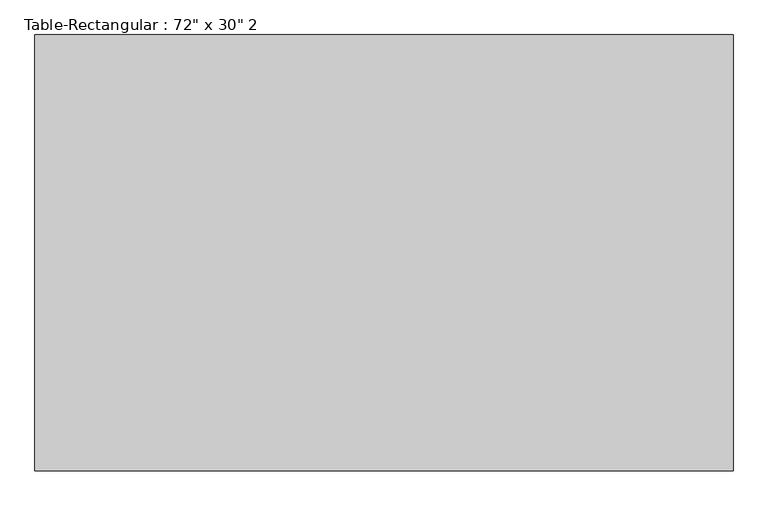
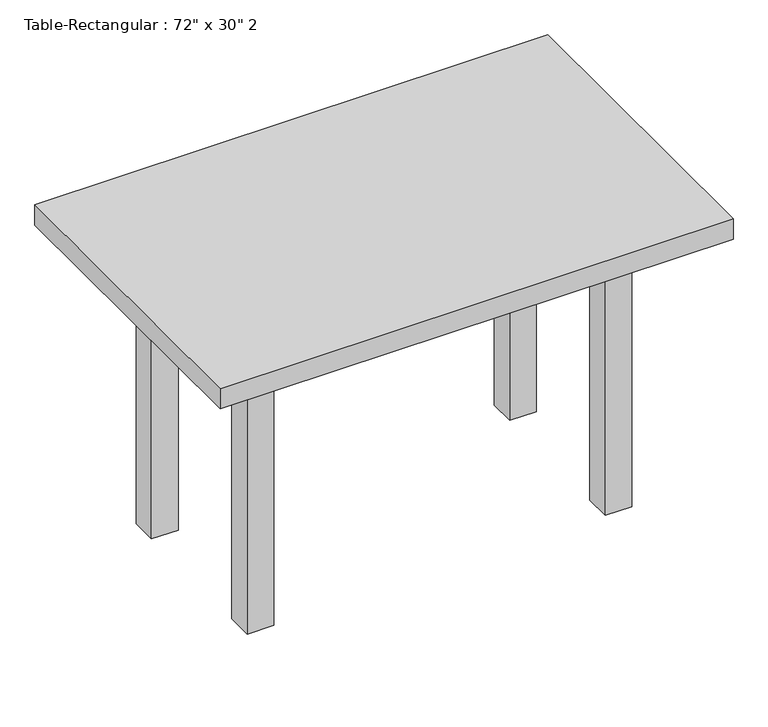
"""IFC4 building model written with IfcOpenShell, lengths in millimetres: furniture geometry."""

from ifc_helpers import new_model, si_unit, frame, origin, origin_with_axes, place, context, project, spatial, polyline, outline, extrude, source, transform, mapped, element, save


def furniture_fc20a73e(model_context):
    return source(origin(), model_context, "Body", "SweptSolid", [
        extrude(outline(polyline([(-393.7, 228.6), (-393.7, 165.1), (-457.2, 165.1), (-457.2, 228.6), (-393.7, 228.6)])), origin_with_axes(), (0.0, 0.0, 1.0), 711.2),
        extrude(outline(polyline([(393.7, 228.6), (457.2, 228.6), (457.2, 165.1), (393.7, 165.1), (393.7, 228.6)])), origin_with_axes(), (0.0, 0.0, 1.0), 711.2),
        extrude(outline(polyline([(-393.7, -228.6), (-457.2, -228.6), (-457.2, -165.1), (-393.7, -165.1), (-393.7, -228.6)])), origin_with_axes(), (0.0, 0.0, 1.0), 711.2),
        extrude(outline(polyline([(393.7, -228.6), (393.7, -165.1), (457.2, -165.1), (457.2, -228.6), (393.7, -228.6)])), origin_with_axes(), (0.0, 0.0, 1.0), 711.2),
        extrude(outline(polyline([(609.6, 381.0), (609.6, -381.0), (-609.6, -381.0), (-609.6, 381.0), (609.6, 381.0)])), frame((0.0, 0.0, 711.2), z_axis=(0.0, 0.0, 1.0), x_axis=(1.0, 0.0, 0.0)), (0.0, 0.0, 1.0), 50.8),
        extrude(outline(polyline([(393.7, 190.5), (393.7, 165.1), (-393.7, 165.1), (-393.7, 190.5), (393.7, 190.5)])), frame((0.0, 0.0, 609.6), z_axis=(0.0, 0.0, 1.0), x_axis=(1.0, 0.0, 0.0)), (0.0, 0.0, 1.0), 101.6),
        extrude(outline(polyline([(393.7, -190.5), (-393.7, -190.5), (-393.7, -165.1), (393.7, -165.1), (393.7, -190.5)])), frame((0.0, 0.0, 609.6), z_axis=(0.0, 0.0, 1.0), x_axis=(1.0, 0.0, 0.0)), (0.0, 0.0, 1.0), 101.6),
        extrude(outline(polyline([(-406.4, -165.1), (-431.8, -165.1), (-431.8, 165.1), (-406.4, 165.1), (-406.4, -165.1)])), frame((0.0, 0.0, 609.6), z_axis=(0.0, 0.0, 1.0), x_axis=(1.0, 0.0, 0.0)), (0.0, 0.0, 1.0), 101.6),
        extrude(outline(polyline([(406.4, -165.1), (406.4, 165.1), (431.8, 165.1), (431.8, -165.1), (406.4, -165.1)])), frame((0.0, 0.0, 609.6), z_axis=(0.0, 0.0, 1.0), x_axis=(1.0, 0.0, 0.0)), (0.0, 0.0, 1.0), 101.6),
    ])


if __name__ == "__main__":
    model = new_model("IFC4")
    model_context = context("Model", 3, world=origin())
    ifc_project = project(units=[si_unit("LENGTHUNIT", "METRE", prefix="MILLI")], contexts=[model_context])
    site = spatial("IfcSite", under=ifc_project)
    building = spatial("IfcBuilding", under=site)
    placement = place(None, origin())
    furniture_shape = furniture_fc20a73e(model_context)
    element("IfcFurniture", 1, ObjectType="Table-Rectangular : 72\" x 30\" 2", at=placement, inside=building, context=model_context, shape_type="MappedRepresentation", body=[
        mapped(furniture_shape, transform((0.0, 0.0, 0.0), x_axis=(1.0, 0.0, 0.0), y_axis=(0.0, 1.0, 0.0), z_axis=(0.0, 0.0, 1.0))),
    ])
    save(model, "model.ifc")

# Revit data of these elements
# Type "Table-Rectangular : 72\" x 30\" 2"
#   Assembly Code = "E2020200"
#   Height = 2' - 6"
#   Length = 4' - 0"
#   Width = 2' - 6"
#   Base Material = Birch
#   Top Material = Birch
#   Default Elevation = 0
# Element 1 (IfcFurniture, "Table-Rectangular : 72\" x 30\" 2")
#   Materials on its faces: "Birch"
# Materials
#   "Birch": class "Wood", colour RGB 224 178 126, transparency 0, Description = "Betula Alleghaniensis", Cost = 0
